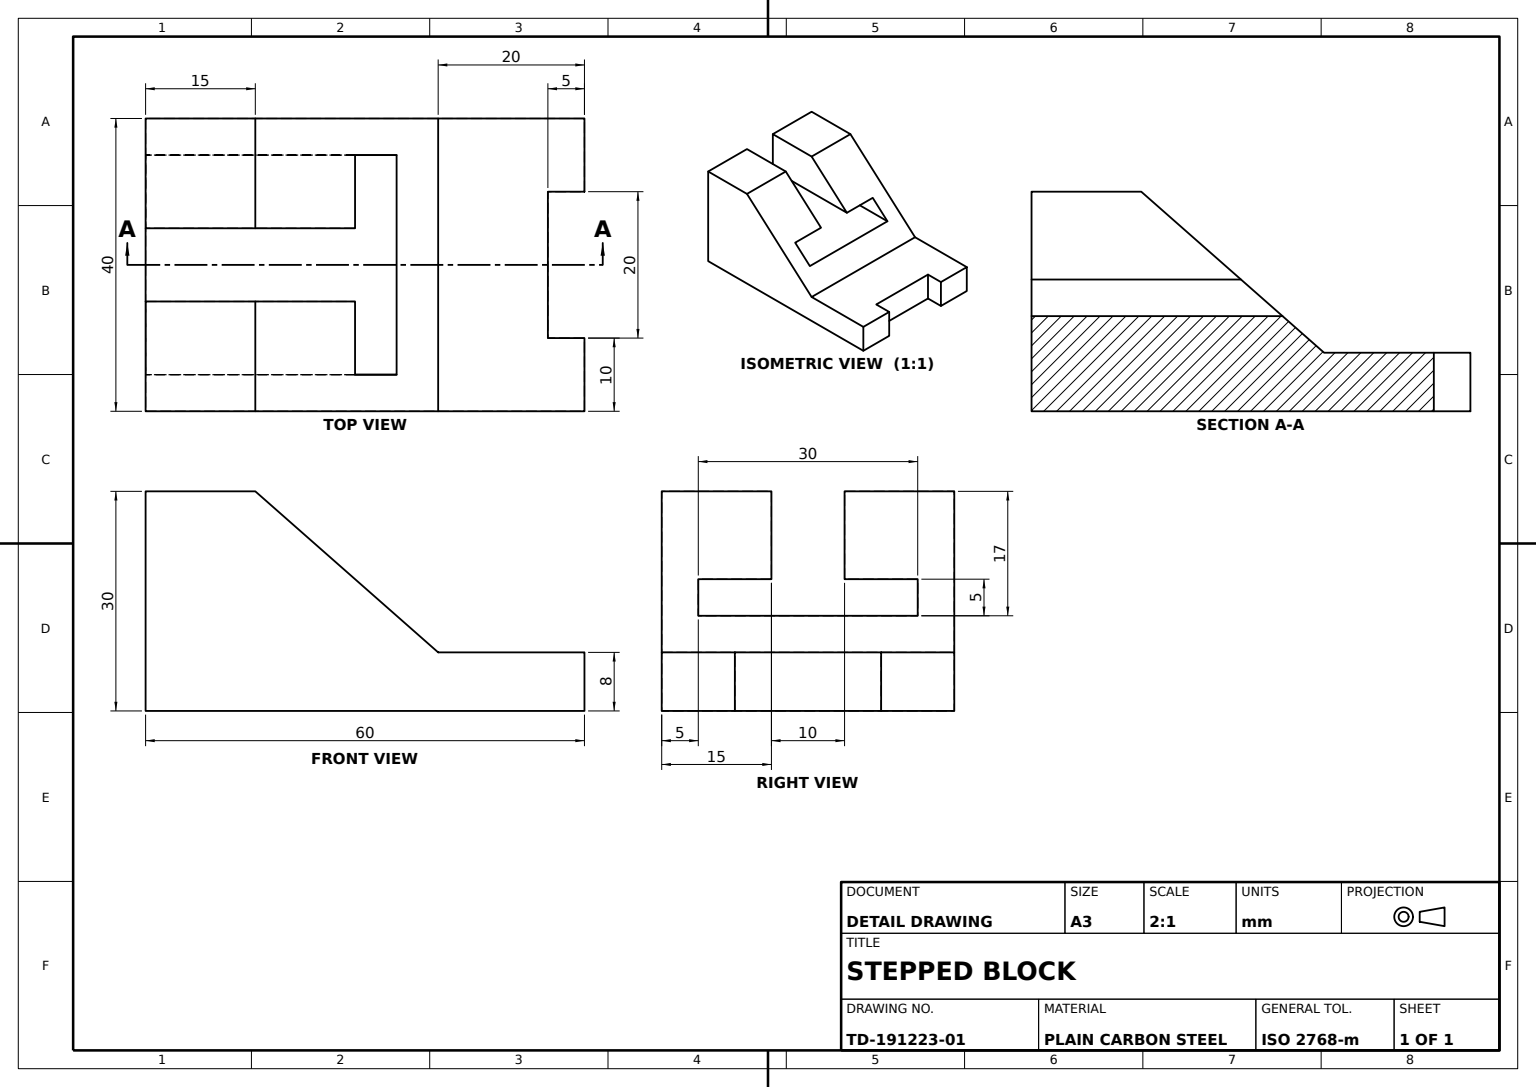
from build123d import *

# Parameters (mm, degrees)
BASE_PLATE_8MM_DEPTH      = 8
UPRIGHT_LOWER_15MM_DEPTH  = 15
UPRIGHT_MIDDLE_15MM_DEPTH = 15
UPRIGHT_TOP_SKETCH_W      = 10
UPRIGHT_TOP_SKETCH_H      = 40
UPRIGHT_TOP_10MM_DEPTH    = 10
SLOPE_CUT_DEPTH           = 40
CENTRE_SLOT_CUT_DEPTH     = 40
FRONT_NOTCH_CUT_DEPTH     = 40


with BuildPart() as part:
    # Base Plate Sketch → Base Plate 8mm (new body)
    with BuildSketch(Plane(origin=(0, 0, 0), x_dir=(1, 0, 0), z_dir=(0, 1, 0))):
        Polygon((0, 0), (20, 0), (20, 60), (-20, 60), (-20, 0), align=None)
    extrude(amount=BASE_PLATE_8MM_DEPTH)

    # Upright Lower Sketch → Upright Lower 15mm (add)
    with BuildSketch(Plane(origin=(20, 0, 0), x_dir=(0, 0, -1), z_dir=(1, 0, 0))):
        Polygon((60, 8), (60, 30), (45, 30), (20, 8), align=None)
    extrude(amount=-UPRIGHT_LOWER_15MM_DEPTH)

    # Upright Middle Sketch → Upright Middle 15mm (add)
    with BuildSketch(Plane.ZY.offset(20)):
        Polygon((-60, 8), (-60, 30), (-45, 30), (-20, 8), align=None)
    extrude(amount=-UPRIGHT_MIDDLE_15MM_DEPTH)

    # Upright Top Sketch → Upright Top 10mm (add)
    with BuildSketch(Plane(origin=(0, 8, 0), x_dir=(1, 0, 0), z_dir=(0, 1, 0))):
        with Locations((0, 40)):
            Rectangle(UPRIGHT_TOP_SKETCH_W, UPRIGHT_TOP_SKETCH_H)
    extrude(amount=UPRIGHT_TOP_10MM_DEPTH)

    # Slope Cut Sketch → Slope Cut (cut)
    with BuildSketch(Plane(origin=(5, 0, 0), x_dir=(0, 0, -1), z_dir=(1, 0, 0))):
        Polygon((20, 8), (20, 18), (31.363636364, 18), align=None)
    extrude(amount=-SLOPE_CUT_DEPTH, mode=Mode.SUBTRACT)

    # Centre Slot Sketch → Centre Slot Cut (cut)
    with BuildSketch(Plane(origin=(0, 0, -60), x_dir=(-1, 0, 0), z_dir=(0, 0, -1))):
        Polygon((0, 13), (15, 13), (15, 18), (-15, 18), (-15, 13), align=None)
    extrude(amount=-CENTRE_SLOT_CUT_DEPTH, mode=Mode.SUBTRACT)

    # Front Notch Sketch → Front Notch Cut (cut)
    with BuildSketch(Plane(origin=(0, 8, 0), x_dir=(1, 0, 0), z_dir=(0, 1, 0))):
        Polygon((0, 5), (10, 5), (10, 0), (-10, 0), (-10, 5), align=None)
    extrude(amount=-FRONT_NOTCH_CUT_DEPTH, mode=Mode.SUBTRACT)


solid = part.part
